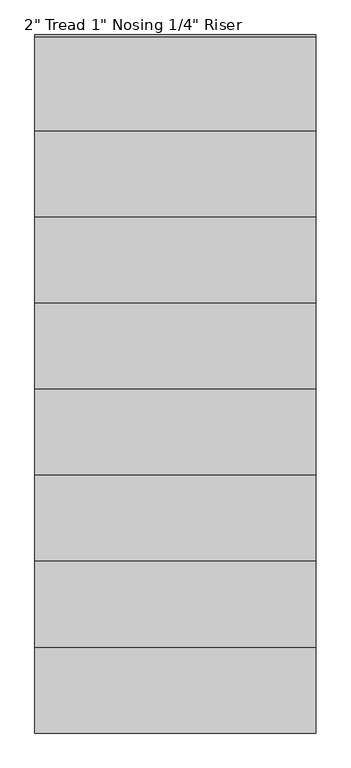
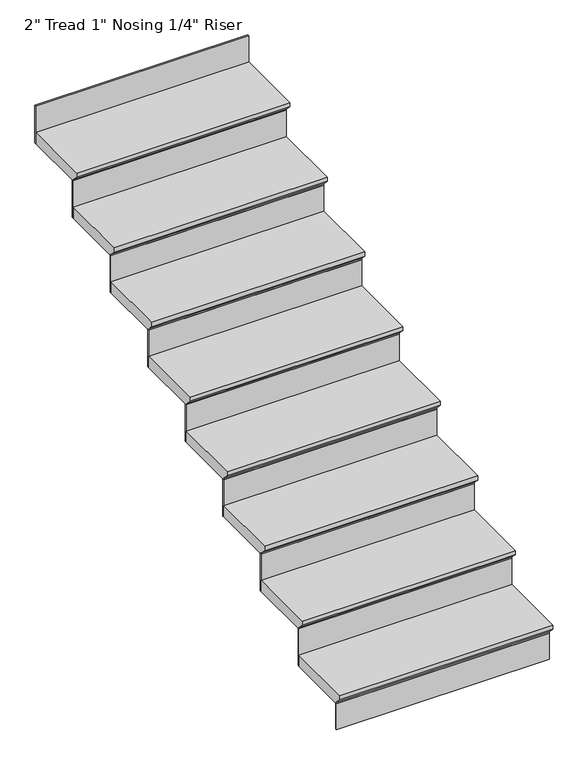
"""IFC4 building model written with IfcOpenShell, lengths in millimetres: stair flight geometry."""

from ifc_helpers import new_model, si_unit, frame, origin, place, context, project, spatial, polyline, outline, extrude, source, transform, mapped, element, save


def stair_flight_8b003f58(model_context):
    return source(origin(), model_context, "Body", "SweptSolid", [
        extrude(outline(polyline([(1930.818583, 1693.3333333), (2235.618583, 1693.3333333), (2235.618583, 1642.5333333), (1956.218583, 1642.5333333), (1956.218583, 1648.8833333), (1930.818583, 1674.2833333), (1930.818583, 1693.3333333)])), frame((-1263.0789517, 0.0, 0.0), z_axis=(1.0, 0.0, 0.0), x_axis=(0.0, 1.0, 0.0)), (0.0, 0.0, 1.0), 914.4),
        extrude(outline(polyline([(-348.6789517, 1962.568583), (-348.6789517, 1956.218583), (-1263.0789517, 1956.218583), (-1263.0789517, 1962.568583), (-348.6789517, 1962.568583)])), frame((0.0, 0.0, 1524.0), z_axis=(0.0, 0.0, 1.0), x_axis=(1.0, 0.0, 0.0)), (0.0, 0.0, 1.0), 118.5333333),
        extrude(outline(polyline([(-348.6789517, 2241.968583), (-348.6789517, 2235.618583), (-1263.0789517, 2235.618583), (-1263.0789517, 2241.968583), (-348.6789517, 2241.968583)])), frame((0.0, 0.0, 1642.5333333), z_axis=(0.0, 0.0, 1.0), x_axis=(1.0, 0.0, 0.0)), (0.0, 0.0, 1.0), 169.3333333),
        extrude(outline(polyline([(2210.218583, 1862.6666667), (2515.018583, 1862.6666667), (2515.018583, 1811.8666667), (2235.618583, 1811.8666667), (2235.618583, 1818.2166667), (2210.218583, 1843.6166667), (2210.218583, 1862.6666667)])), frame((-1263.0789517, 0.0, 0.0), z_axis=(1.0, 0.0, 0.0), x_axis=(0.0, 1.0, 0.0)), (0.0, 0.0, 1.0), 914.4),
        extrude(outline(polyline([(-348.6789517, 2521.368583), (-348.6789517, 2515.018583), (-1263.0789517, 2515.018583), (-1263.0789517, 2521.368583), (-348.6789517, 2521.368583)])), frame((0.0, 0.0, 1811.8666667), z_axis=(0.0, 0.0, 1.0), x_axis=(1.0, 0.0, 0.0)), (0.0, 0.0, 1.0), 169.3333333),
        extrude(outline(polyline([(2489.618583, 2032.0), (2794.418583, 2032.0), (2794.418583, 1981.2), (2515.018583, 1981.2), (2515.018583, 1987.55), (2489.618583, 2012.95), (2489.618583, 2032.0)])), frame((-1263.0789517, 0.0, 0.0), z_axis=(1.0, 0.0, 0.0), x_axis=(0.0, 1.0, 0.0)), (0.0, 0.0, 1.0), 914.4),
        extrude(outline(polyline([(-348.6789517, 2800.768583), (-348.6789517, 2794.418583), (-1263.0789517, 2794.418583), (-1263.0789517, 2800.768583), (-348.6789517, 2800.768583)])), frame((0.0, 0.0, 1981.2), z_axis=(0.0, 0.0, 1.0), x_axis=(1.0, 0.0, 0.0)), (0.0, 0.0, 1.0), 169.3333333),
        extrude(outline(polyline([(2769.018583, 2201.3333333), (3073.818583, 2201.3333333), (3073.818583, 2150.5333333), (2794.418583, 2150.5333333), (2794.418583, 2156.8833333), (2769.018583, 2182.2833333), (2769.018583, 2201.3333333)])), frame((-1263.0789517, 0.0, 0.0), z_axis=(1.0, 0.0, 0.0), x_axis=(0.0, 1.0, 0.0)), (0.0, 0.0, 1.0), 914.4),
        extrude(outline(polyline([(-348.6789517, 3080.168583), (-348.6789517, 3073.818583), (-1263.0789517, 3073.818583), (-1263.0789517, 3080.168583), (-348.6789517, 3080.168583)])), frame((0.0, 0.0, 2150.5333333), z_axis=(0.0, 0.0, 1.0), x_axis=(1.0, 0.0, 0.0)), (0.0, 0.0, 1.0), 169.3333333),
        extrude(outline(polyline([(3048.418583, 2370.6666667), (3353.218583, 2370.6666667), (3353.218583, 2319.8666667), (3073.818583, 2319.8666667), (3073.818583, 2326.2166667), (3048.418583, 2351.6166667), (3048.418583, 2370.6666667)])), frame((-1263.0789517, 0.0, 0.0), z_axis=(1.0, 0.0, 0.0), x_axis=(0.0, 1.0, 0.0)), (0.0, 0.0, 1.0), 914.4),
        extrude(outline(polyline([(-348.6789517, 3359.568583), (-348.6789517, 3353.218583), (-1263.0789517, 3353.218583), (-1263.0789517, 3359.568583), (-348.6789517, 3359.568583)])), frame((0.0, 0.0, 2319.8666667), z_axis=(0.0, 0.0, 1.0), x_axis=(1.0, 0.0, 0.0)), (0.0, 0.0, 1.0), 169.3333333),
        extrude(outline(polyline([(3327.818583, 2540.0), (3632.618583, 2540.0), (3632.618583, 2489.2), (3353.218583, 2489.2), (3353.218583, 2495.55), (3327.818583, 2520.95), (3327.818583, 2540.0)])), frame((-1263.0789517, 0.0, 0.0), z_axis=(1.0, 0.0, 0.0), x_axis=(0.0, 1.0, 0.0)), (0.0, 0.0, 1.0), 914.4),
        extrude(outline(polyline([(-348.6789517, 3638.968583), (-348.6789517, 3632.618583), (-1263.0789517, 3632.618583), (-1263.0789517, 3638.968583), (-348.6789517, 3638.968583)])), frame((0.0, 0.0, 2489.2), z_axis=(0.0, 0.0, 1.0), x_axis=(1.0, 0.0, 0.0)), (0.0, 0.0, 1.0), 169.3333333),
        extrude(outline(polyline([(3607.218583, 2709.3333333), (3912.018583, 2709.3333333), (3912.018583, 2658.5333333), (3632.618583, 2658.5333333), (3632.618583, 2664.8833333), (3607.218583, 2690.2833333), (3607.218583, 2709.3333333)])), frame((-1263.0789517, 0.0, 0.0), z_axis=(1.0, 0.0, 0.0), x_axis=(0.0, 1.0, 0.0)), (0.0, 0.0, 1.0), 914.4),
        extrude(outline(polyline([(-348.6789517, 3918.368583), (-348.6789517, 3912.018583), (-1263.0789517, 3912.018583), (-1263.0789517, 3918.368583), (-348.6789517, 3918.368583)])), frame((0.0, 0.0, 2658.5333333), z_axis=(0.0, 0.0, 1.0), x_axis=(1.0, 0.0, 0.0)), (0.0, 0.0, 1.0), 169.3333333),
        extrude(outline(polyline([(-348.6789517, 4197.768583), (-348.6789517, 4191.418583), (-1263.0789517, 4191.418583), (-1263.0789517, 4197.768583), (-348.6789517, 4197.768583)])), frame((0.0, 0.0, 2827.8666667), z_axis=(0.0, 0.0, 1.0), x_axis=(1.0, 0.0, 0.0)), (0.0, 0.0, 1.0), 169.3333333),
        extrude(outline(polyline([(3886.618583, 2878.6666667), (4191.418583, 2878.6666667), (4191.418583, 2827.8666667), (3912.018583, 2827.8666667), (3912.018583, 2834.2166667), (3886.618583, 2859.6166667), (3886.618583, 2878.6666667)])), frame((-1263.0789517, 0.0, 0.0), z_axis=(1.0, 0.0, 0.0), x_axis=(0.0, 1.0, 0.0)), (0.0, 0.0, 1.0), 914.4),
    ])


if __name__ == "__main__":
    model = new_model("IFC4")
    model_context = context("Model", 3, world=origin())
    ifc_project = project(units=[si_unit("LENGTHUNIT", "METRE", prefix="MILLI")], contexts=[model_context])
    site = spatial("IfcSite", under=ifc_project)
    building = spatial("IfcBuilding", under=site)
    placement = place(None, origin())
    stair_flight_shape = stair_flight_8b003f58(model_context)
    element("IfcStairFlight", 1, ObjectType="2\" Tread 1\" Nosing 1/4\" Riser", at=placement, inside=building, context=model_context, shape_type="MappedRepresentation", body=[
        mapped(stair_flight_shape, transform((0.0, 0.0, 0.0), x_axis=(1.0, 0.0, 0.0), y_axis=(0.0, 1.0, 0.0), z_axis=(0.0, 0.0, 1.0))),
    ])
    save(model, "model.ifc")
